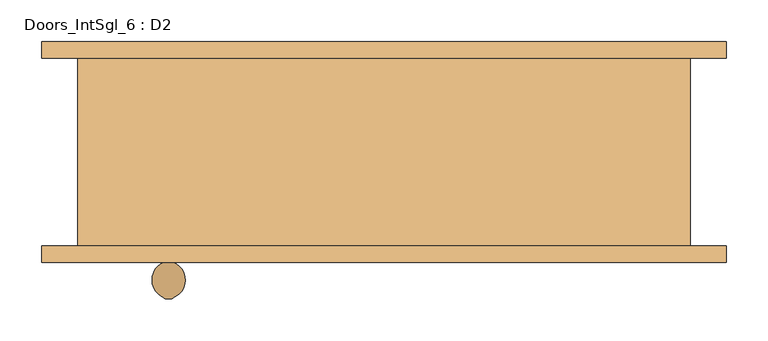
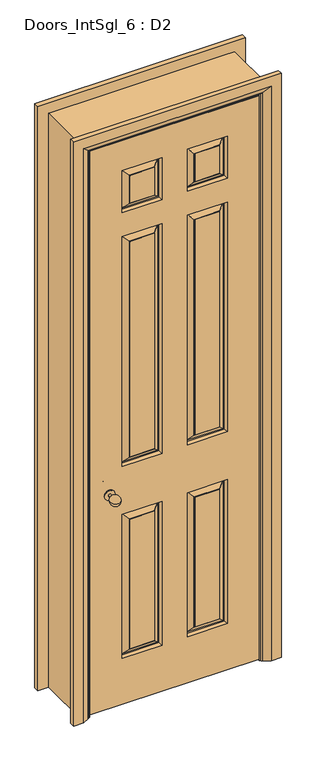
"""IFC4 building model written with IfcOpenShell, lengths in millimetres: door geometry, Doors_IntSgl_6 : D2."""

from ifc_helpers import new_model, si_unit, point, frame, origin, place, context, project, spatial, polyline, circle_curve, ellipse_curve, trimmed, outline, extrude, faceted_brep, source, transform, mapped, element, save
from ifc_brep_helpers import plane_surface, cylinder_surface, revolved_surface, advanced_brep


def doors_intsgl_6_d2_0bf64c77(model_context):
    return source(origin(), model_context, "Body", "SolidModel", [
        advanced_brep(
        [(-253.0, -55.5, 900.0), (-263.0, -55.5, 900.0), (-258.0, -11.062589, 900.0), (-253.0, -70.5, 900.0), (-263.0, -70.5, 900.0), (-278.0, -74.5, 900.0), (-238.0, -74.5, 900.0), (-278.0, -70.5, 900.0), (-238.0, -70.5, 900.0)],
        [
            (0, 1, circle_curve(frame((-258.0, -55.5, 900.0), z_axis=(0.0, 1.0, 0.0), x_axis=(-1.0, 0.0, 0.0)), 5.0)),
            (1, 2, circle_curve(frame((-254.8115138, -33.9213505, 900.0), z_axis=(0.0, 0.0, -1.0), x_axis=(0.0, -1.0, 0.0)), 23.0800654)),
            (2, 0, circle_curve(frame((-261.1884862, -33.9213505, 900.0), z_axis=(0.0, 0.0, -1.0), x_axis=(0.0, -1.0, 0.0)), 23.0800654)),
            (1, 0, circle_curve(frame((-258.0, -55.5, 900.0), z_axis=(0.0, 1.0, 0.0), x_axis=(-1.0, 0.0, 0.0)), 5.0)),
            (0, 3),
            (3, 4, circle_curve(frame((-258.0, -70.5, 900.0), z_axis=(0.0, 1.0, 0.0), x_axis=(-1.0, 0.0, 0.0)), 5.0)),
            (4, 1),
            (4, 3, circle_curve(frame((-258.0, -70.5, 900.0), z_axis=(0.0, 1.0, 0.0), x_axis=(-1.0, 0.0, 0.0)), 5.0)),
            (5, 6, circle_curve(frame((-258.0, -74.5, 900.0), z_axis=(0.0, -1.0, 0.0), x_axis=(1.0, 0.0, 0.0)), 20.0)),
            (6, 5, circle_curve(frame((-258.0, -74.5, 900.0), z_axis=(0.0, -1.0, 0.0), x_axis=(1.0, 0.0, 0.0)), 20.0)),
            (7, 8, circle_curve(frame((-258.0, -70.5, 900.0), z_axis=(0.0, 1.0, 0.0), x_axis=(1.0, 0.0, 0.0)), 20.0)),
            (8, 7, circle_curve(frame((-258.0, -70.5, 900.0), z_axis=(0.0, 1.0, 0.0), x_axis=(1.0, 0.0, 0.0)), 20.0)),
            (5, 7),
            (8, 6),
        ],
        [
            revolved_surface(trimmed(ellipse_curve(frame((-254.8115138, -33.9213505, 900.0), z_axis=(0.0, 0.0, 1.0), x_axis=(0.0, -1.0, 0.0)), 23.0800654, 23.0800654), [point((-258.0, -11.062589, 900.0))], [point((-263.0, -55.5, 900.0))], True, "CARTESIAN"), (-258.0, -70.5, 900.0), (0.0, -1.0, 0.0)),
            cylinder_surface(frame((-258.0, -70.5, 900.0), z_axis=(0.0, -1.0, 0.0), x_axis=(-1.0, 0.0, 0.0)), 5.0),
            plane_surface(frame((-238.0, -74.5, 900.0), z_axis=(0.0, -1.0, 0.0), x_axis=(0.0, 0.0, 1.0))),
            plane_surface(frame((-238.0, -70.5, 900.0), z_axis=(0.0, 1.0, 0.0), x_axis=(0.0, 0.0, -1.0))),
            cylinder_surface(frame((-258.0, -70.5, 900.0), z_axis=(0.0, -1.0, 0.0), x_axis=(1.0, 0.0, 0.0)), 20.0),
        ],
        [
            (0, [[1, 2, 3]]),
            (0, [[-2, 4, -3]]),
            (1, [[-1, 5, 6, 7]]),
            (1, [[-4, -7, 8, -5]]),
            (2, [[9, 10]]),
            (3, [[11, 12], [-6, -8]]),
            (4, [[-9, 13, -12, 14]]),
            (4, [[-10, -14, -11, -13]]),
        ],
    ),
        advanced_brep(
        [(-253.0, -131.5, 900.0), (-258.0, -175.937411, 900.0), (-263.0, -131.5, 900.0), (-263.0, -116.5, 900.0), (-253.0, -116.5, 900.0), (-278.0, -112.5, 900.0), (-238.0, -112.5, 900.0), (-278.0, -116.5, 900.0), (-238.0, -116.5, 900.0)],
        [
            (0, 1, circle_curve(frame((-261.1884862, -153.0786495, 900.0), z_axis=(0.0, 0.0, -1.0), x_axis=(0.0, 1.0, 0.0)), 23.0800654)),
            (1, 2, circle_curve(frame((-254.8115138, -153.0786495, 900.0), z_axis=(0.0, 0.0, -1.0), x_axis=(0.0, 1.0, 0.0)), 23.0800654)),
            (2, 0, circle_curve(frame((-258.0, -131.5, 900.0), z_axis=(0.0, -1.0, 0.0), x_axis=(-1.0, 0.0, 0.0)), 5.0)),
            (0, 2, circle_curve(frame((-258.0, -131.5, 900.0), z_axis=(0.0, -1.0, 0.0), x_axis=(-1.0, 0.0, 0.0)), 5.0)),
            (2, 3),
            (3, 4, circle_curve(frame((-258.0, -116.5, 900.0), z_axis=(0.0, -1.0, 0.0), x_axis=(-1.0, 0.0, 0.0)), 5.0)),
            (4, 0),
            (4, 3, circle_curve(frame((-258.0, -116.5, 900.0), z_axis=(0.0, -1.0, 0.0), x_axis=(-1.0, 0.0, 0.0)), 5.0)),
            (5, 6, circle_curve(frame((-258.0, -112.5, 900.0), z_axis=(0.0, 1.0, 0.0), x_axis=(1.0, 0.0, 0.0)), 20.0)),
            (6, 5, circle_curve(frame((-258.0, -112.5, 900.0), z_axis=(0.0, 1.0, 0.0), x_axis=(1.0, 0.0, 0.0)), 20.0)),
            (7, 8, circle_curve(frame((-258.0, -116.5, 900.0), z_axis=(0.0, -1.0, 0.0), x_axis=(1.0, 0.0, 0.0)), 20.0)),
            (8, 7, circle_curve(frame((-258.0, -116.5, 900.0), z_axis=(0.0, -1.0, 0.0), x_axis=(1.0, 0.0, 0.0)), 20.0)),
            (6, 8),
            (7, 5),
        ],
        [
            revolved_surface(trimmed(ellipse_curve(frame((-254.8115138, -153.0786495, 900.0), z_axis=(0.0, 0.0, -1.0), x_axis=(0.0, 1.0, 0.0)), 23.0800654, 23.0800654), [point((-258.0, -175.937411, 900.0))], [point((-263.0, -131.5, 900.0))], True, "CARTESIAN"), (-258.0, -116.5, 900.0), (0.0, 1.0, 0.0)),
            cylinder_surface(frame((-258.0, -116.5, 900.0), z_axis=(0.0, 1.0, 0.0), x_axis=(-1.0, 0.0, 0.0)), 5.0),
            plane_surface(frame((-238.0, -112.5, 900.0), z_axis=(0.0, 1.0, 0.0), x_axis=(0.0, 0.0, 1.0))),
            plane_surface(frame((-238.0, -116.5, 900.0), z_axis=(0.0, -1.0, 0.0), x_axis=(0.0, 0.0, -1.0))),
            cylinder_surface(frame((-258.0, -116.5, 900.0), z_axis=(0.0, 1.0, 0.0), x_axis=(1.0, 0.0, 0.0)), 20.0),
        ],
        [
            (0, [[1, 2, 3]]),
            (0, [[-1, 4, -2]]),
            (1, [[5, 6, 7, -3]]),
            (1, [[-7, 8, -5, -4]]),
            (2, [[9, 10]]),
            (3, [[11, 12], [-8, -6]]),
            (4, [[13, -11, 14, -10]]),
            (4, [[-14, -12, -13, -9]]),
        ],
    ),
        faceted_brep([(-333.0, -74.5, 2358.0), (333.0, -74.5, 2358.0), (333.0, -74.5, 8.0), (-333.0, -74.5, 8.0), (-50.0, -74.5, 800.0), (-208.0, -74.5, 800.0), (-208.0, -74.5, 200.0), (-50.0, -74.5, 200.0), (208.0, -74.5, 800.0), (50.0, -74.5, 800.0), (50.0, -74.5, 200.0), (208.0, -74.5, 200.0), (-50.0, -74.5, 1958.0), (-208.0, -74.5, 1958.0), (-208.0, -74.5, 1000.0), (-50.0, -74.5, 1000.0), (208.0, -74.5, 1958.0), (50.0, -74.5, 1958.0), (50.0, -74.5, 1000.0), (208.0, -74.5, 1000.0), (-50.0, -74.5, 2233.0), (-208.0, -74.5, 2233.0), (-208.0, -74.5, 2058.0), (-50.0, -74.5, 2058.0), (208.0, -74.5, 2233.0), (50.0, -74.5, 2233.0), (50.0, -74.5, 2058.0), (208.0, -74.5, 2058.0), (-80.0, -74.5, 230.0), (-178.0, -74.5, 230.0), (-178.0, -74.5, 770.0), (-80.0, -74.5, 770.0), (178.0, -74.5, 230.0), (80.0, -74.5, 230.0), (80.0, -74.5, 770.0), (178.0, -74.5, 770.0), (-80.0, -74.5, 1030.0), (-178.0, -74.5, 1030.0), (-178.0, -74.5, 1928.0), (-80.0, -74.5, 1928.0), (178.0, -74.5, 1030.0), (80.0, -74.5, 1030.0), (80.0, -74.5, 1928.0), (178.0, -74.5, 1928.0), (-80.0, -74.5, 2088.0), (-178.0, -74.5, 2088.0), (-178.0, -74.5, 2203.0), (-80.0, -74.5, 2203.0), (178.0, -74.5, 2088.0), (80.0, -74.5, 2088.0), (80.0, -74.5, 2203.0), (178.0, -74.5, 2203.0), (-333.0, -112.5, 2358.0), (-333.0, -112.5, 8.0), (333.0, -112.5, 8.0), (333.0, -112.5, 2358.0), (50.0, -112.5, 800.0), (208.0, -112.5, 800.0), (208.0, -112.5, 200.0), (50.0, -112.5, 200.0), (-208.0, -112.5, 800.0), (-50.0, -112.5, 800.0), (-50.0, -112.5, 200.0), (-208.0, -112.5, 200.0), (50.0, -112.5, 1958.0), (208.0, -112.5, 1958.0), (208.0, -112.5, 1000.0), (50.0, -112.5, 1000.0), (-208.0, -112.5, 1958.0), (-50.0, -112.5, 1958.0), (-50.0, -112.5, 1000.0), (-208.0, -112.5, 1000.0), (50.0, -112.5, 2233.0), (208.0, -112.5, 2233.0), (208.0, -112.5, 2058.0), (50.0, -112.5, 2058.0), (-208.0, -112.5, 2233.0), (-50.0, -112.5, 2233.0), (-50.0, -112.5, 2058.0), (-208.0, -112.5, 2058.0), (80.0, -112.5, 230.0), (178.0, -112.5, 230.0), (178.0, -112.5, 770.0), (80.0, -112.5, 770.0), (-178.0, -112.5, 230.0), (-80.0, -112.5, 230.0), (-80.0, -112.5, 770.0), (-178.0, -112.5, 770.0), (80.0, -112.5, 1030.0), (178.0, -112.5, 1030.0), (178.0, -112.5, 1928.0), (80.0, -112.5, 1928.0), (-178.0, -112.5, 1030.0), (-80.0, -112.5, 1030.0), (-80.0, -112.5, 1928.0), (-178.0, -112.5, 1928.0), (80.0, -112.5, 2088.0), (178.0, -112.5, 2088.0), (178.0, -112.5, 2203.0), (80.0, -112.5, 2203.0), (-178.0, -112.5, 2088.0), (-80.0, -112.5, 2088.0), (-80.0, -112.5, 2203.0), (-178.0, -112.5, 2203.0), (80.0, -111.5, 230.0), (80.0, -111.5, 770.0), (58.0, -97.5, 208.0), (78.0, -111.5, 228.0), (78.0, -111.5, 772.0), (58.0, -97.5, 792.0), (53.0, -97.5, 203.0), (53.0, -97.5, 797.0), (178.0, -111.5, 770.0), (180.0, -111.5, 772.0), (200.0, -97.5, 792.0), (205.0, -97.5, 797.0), (178.0, -111.5, 230.0), (180.0, -111.5, 228.0), (200.0, -97.5, 208.0), (205.0, -97.5, 203.0), (-178.0, -111.5, 230.0), (-178.0, -111.5, 770.0), (-200.0, -97.5, 208.0), (-180.0, -111.5, 228.0), (-180.0, -111.5, 772.0), (-200.0, -97.5, 792.0), (-205.0, -97.5, 203.0), (-205.0, -97.5, 797.0), (-80.0, -111.5, 770.0), (-78.0, -111.5, 772.0), (-58.0, -97.5, 792.0), (-53.0, -97.5, 797.0), (-80.0, -111.5, 230.0), (-78.0, -111.5, 228.0), (-58.0, -97.5, 208.0), (-53.0, -97.5, 203.0), (80.0, -111.5, 1030.0), (80.0, -111.5, 1928.0), (58.0, -97.5, 1008.0), (78.0, -111.5, 1028.0), (78.0, -111.5, 1930.0), (58.0, -97.5, 1950.0), (53.0, -97.5, 1003.0), (53.0, -97.5, 1955.0), (178.0, -111.5, 1928.0), (180.0, -111.5, 1930.0), (200.0, -97.5, 1950.0), (205.0, -97.5, 1955.0), (178.0, -111.5, 1030.0), (180.0, -111.5, 1028.0), (200.0, -97.5, 1008.0), (205.0, -97.5, 1003.0), (-178.0, -111.5, 1030.0), (-178.0, -111.5, 1928.0), (-200.0, -97.5, 1008.0), (-180.0, -111.5, 1028.0), (-180.0, -111.5, 1930.0), (-200.0, -97.5, 1950.0), (-205.0, -97.5, 1003.0), (-205.0, -97.5, 1955.0), (-80.0, -111.5, 1928.0), (-78.0, -111.5, 1930.0), (-58.0, -97.5, 1950.0), (-53.0, -97.5, 1955.0), (-80.0, -111.5, 1030.0), (-78.0, -111.5, 1028.0), (-58.0, -97.5, 1008.0), (-53.0, -97.5, 1003.0), (80.0, -111.5, 2088.0), (80.0, -111.5, 2203.0), (58.0, -97.5, 2066.0), (78.0, -111.5, 2086.0), (78.0, -111.5, 2205.0), (58.0, -97.5, 2225.0), (53.0, -97.5, 2061.0), (53.0, -97.5, 2230.0), (178.0, -111.5, 2203.0), (180.0, -111.5, 2205.0), (200.0, -97.5, 2225.0), (205.0, -97.5, 2230.0), (178.0, -111.5, 2088.0), (180.0, -111.5, 2086.0), (200.0, -97.5, 2066.0), (205.0, -97.5, 2061.0), (-178.0, -111.5, 2088.0), (-178.0, -111.5, 2203.0), (-200.0, -97.5, 2066.0), (-180.0, -111.5, 2086.0), (-180.0, -111.5, 2205.0), (-200.0, -97.5, 2225.0), (-205.0, -97.5, 2061.0), (-205.0, -97.5, 2230.0), (-80.0, -111.5, 2203.0), (-78.0, -111.5, 2205.0), (-58.0, -97.5, 2225.0), (-53.0, -97.5, 2230.0), (-80.0, -111.5, 2088.0), (-78.0, -111.5, 2086.0), (-58.0, -97.5, 2066.0), (-53.0, -97.5, 2061.0), (-80.0, -75.5, 230.0), (-80.0, -75.5, 770.0), (-58.0, -89.5, 208.0), (-78.0, -75.5, 228.0), (-78.0, -75.5, 772.0), (-58.0, -89.5, 792.0), (-53.0, -89.5, 203.0), (-53.0, -89.5, 797.0), (-178.0, -75.5, 770.0), (-180.0, -75.5, 772.0), (-200.0, -89.5, 792.0), (-205.0, -89.5, 797.0), (-178.0, -75.5, 230.0), (-180.0, -75.5, 228.0), (-200.0, -89.5, 208.0), (-205.0, -89.5, 203.0), (178.0, -75.5, 230.0), (178.0, -75.5, 770.0), (200.0, -89.5, 208.0), (180.0, -75.5, 228.0), (180.0, -75.5, 772.0), (200.0, -89.5, 792.0), (205.0, -89.5, 203.0), (205.0, -89.5, 797.0), (80.0, -75.5, 770.0), (78.0, -75.5, 772.0), (58.0, -89.5, 792.0), (53.0, -89.5, 797.0), (80.0, -75.5, 230.0), (78.0, -75.5, 228.0), (58.0, -89.5, 208.0), (53.0, -89.5, 203.0), (-80.0, -75.5, 1030.0), (-80.0, -75.5, 1928.0), (-58.0, -89.5, 1008.0), (-78.0, -75.5, 1028.0), (-78.0, -75.5, 1930.0), (-58.0, -89.5, 1950.0), (-53.0, -89.5, 1003.0), (-53.0, -89.5, 1955.0), (-178.0, -75.5, 1928.0), (-180.0, -75.5, 1930.0), (-200.0, -89.5, 1950.0), (-205.0, -89.5, 1955.0), (-178.0, -75.5, 1030.0), (-180.0, -75.5, 1028.0), (-200.0, -89.5, 1008.0), (-205.0, -89.5, 1003.0), (178.0, -75.5, 1030.0), (178.0, -75.5, 1928.0), (200.0, -89.5, 1008.0), (180.0, -75.5, 1028.0), (180.0, -75.5, 1930.0), (200.0, -89.5, 1950.0), (205.0, -89.5, 1003.0), (205.0, -89.5, 1955.0), (80.0, -75.5, 1928.0), (78.0, -75.5, 1930.0), (58.0, -89.5, 1950.0), (53.0, -89.5, 1955.0), (80.0, -75.5, 1030.0), (78.0, -75.5, 1028.0), (58.0, -89.5, 1008.0), (53.0, -89.5, 1003.0), (-80.0, -75.5, 2088.0), (-80.0, -75.5, 2203.0), (-58.0, -89.5, 2066.0), (-78.0, -75.5, 2086.0), (-78.0, -75.5, 2205.0), (-58.0, -89.5, 2225.0), (-53.0, -89.5, 2061.0), (-53.0, -89.5, 2230.0), (-178.0, -75.5, 2203.0), (-180.0, -75.5, 2205.0), (-200.0, -89.5, 2225.0), (-205.0, -89.5, 2230.0), (-178.0, -75.5, 2088.0), (-180.0, -75.5, 2086.0), (-200.0, -89.5, 2066.0), (-205.0, -89.5, 2061.0), (178.0, -75.5, 2088.0), (178.0, -75.5, 2203.0), (200.0, -89.5, 2066.0), (180.0, -75.5, 2086.0), (180.0, -75.5, 2205.0), (200.0, -89.5, 2225.0), (205.0, -89.5, 2061.0), (205.0, -89.5, 2230.0), (80.0, -75.5, 2203.0), (78.0, -75.5, 2205.0), (58.0, -89.5, 2225.0), (53.0, -89.5, 2230.0), (80.0, -75.5, 2088.0), (78.0, -75.5, 2086.0), (58.0, -89.5, 2066.0), (53.0, -89.5, 2061.0)], [[[0, 1, 2, 3], [4, 5, 6, 7], [8, 9, 10, 11], [12, 13, 14, 15], [16, 17, 18, 19], [20, 21, 22, 23], [24, 25, 26, 27]], [[28, 29, 30, 31]], [[32, 33, 34, 35]], [[36, 37, 38, 39]], [[40, 41, 42, 43]], [[44, 45, 46, 47]], [[48, 49, 50, 51]], [[52, 53, 54, 55], [56, 57, 58, 59], [60, 61, 62, 63], [64, 65, 66, 67], [68, 69, 70, 71], [72, 73, 74, 75], [76, 77, 78, 79]], [[80, 81, 82, 83]], [[84, 85, 86, 87]], [[88, 89, 90, 91]], [[92, 93, 94, 95]], [[96, 97, 98, 99]], [[100, 101, 102, 103]], [[3, 53, 52, 0]], [[2, 54, 53, 3]], [[1, 55, 54, 2]], [[0, 52, 55, 1]], [[104, 80, 83, 105]], [[106, 107, 108, 109]], [[56, 59, 110, 111]], [[83, 82, 112, 105]], [[108, 113, 114, 109]], [[111, 115, 57, 56]], [[82, 81, 116, 112]], [[113, 117, 118, 114]], [[115, 119, 58, 57]], [[104, 116, 81, 80]], [[107, 117, 113, 108], [105, 112, 116, 104]], [[106, 118, 117, 107]], [[110, 119, 115, 111], [109, 114, 118, 106]], [[59, 58, 119, 110]], [[120, 84, 87, 121]], [[122, 123, 124, 125]], [[60, 63, 126, 127]], [[87, 86, 128, 121]], [[124, 129, 130, 125]], [[127, 131, 61, 60]], [[86, 85, 132, 128]], [[129, 133, 134, 130]], [[131, 135, 62, 61]], [[120, 132, 85, 84]], [[123, 133, 129, 124], [121, 128, 132, 120]], [[122, 134, 133, 123]], [[126, 135, 131, 127], [125, 130, 134, 122]], [[63, 62, 135, 126]], [[136, 88, 91, 137]], [[138, 139, 140, 141]], [[64, 67, 142, 143]], [[91, 90, 144, 137]], [[140, 145, 146, 141]], [[143, 147, 65, 64]], [[90, 89, 148, 144]], [[145, 149, 150, 146]], [[147, 151, 66, 65]], [[136, 148, 89, 88]], [[139, 149, 145, 140], [137, 144, 148, 136]], [[138, 150, 149, 139]], [[142, 151, 147, 143], [141, 146, 150, 138]], [[67, 66, 151, 142]], [[152, 92, 95, 153]], [[154, 155, 156, 157]], [[68, 71, 158, 159]], [[95, 94, 160, 153]], [[156, 161, 162, 157]], [[159, 163, 69, 68]], [[94, 93, 164, 160]], [[161, 165, 166, 162]], [[163, 167, 70, 69]], [[152, 164, 93, 92]], [[155, 165, 161, 156], [153, 160, 164, 152]], [[154, 166, 165, 155]], [[158, 167, 163, 159], [157, 162, 166, 154]], [[71, 70, 167, 158]], [[168, 96, 99, 169]], [[170, 171, 172, 173]], [[72, 75, 174, 175]], [[99, 98, 176, 169]], [[172, 177, 178, 173]], [[175, 179, 73, 72]], [[98, 97, 180, 176]], [[177, 181, 182, 178]], [[179, 183, 74, 73]], [[168, 180, 97, 96]], [[171, 181, 177, 172], [169, 176, 180, 168]], [[170, 182, 181, 171]], [[174, 183, 179, 175], [173, 178, 182, 170]], [[75, 74, 183, 174]], [[184, 100, 103, 185]], [[186, 187, 188, 189]], [[76, 79, 190, 191]], [[103, 102, 192, 185]], [[188, 193, 194, 189]], [[191, 195, 77, 76]], [[102, 101, 196, 192]], [[193, 197, 198, 194]], [[195, 199, 78, 77]], [[184, 196, 101, 100]], [[187, 197, 193, 188], [185, 192, 196, 184]], [[186, 198, 197, 187]], [[190, 199, 195, 191], [189, 194, 198, 186]], [[79, 78, 199, 190]], [[200, 28, 31, 201]], [[202, 203, 204, 205]], [[4, 7, 206, 207]], [[31, 30, 208, 201]], [[204, 209, 210, 205]], [[207, 211, 5, 4]], [[30, 29, 212, 208]], [[209, 213, 214, 210]], [[211, 215, 6, 5]], [[200, 212, 29, 28]], [[203, 213, 209, 204], [201, 208, 212, 200]], [[202, 214, 213, 203]], [[206, 215, 211, 207], [205, 210, 214, 202]], [[7, 6, 215, 206]], [[216, 32, 35, 217]], [[218, 219, 220, 221]], [[8, 11, 222, 223]], [[35, 34, 224, 217]], [[220, 225, 226, 221]], [[223, 227, 9, 8]], [[34, 33, 228, 224]], [[225, 229, 230, 226]], [[227, 231, 10, 9]], [[216, 228, 33, 32]], [[219, 229, 225, 220], [217, 224, 228, 216]], [[218, 230, 229, 219]], [[222, 231, 227, 223], [221, 226, 230, 218]], [[11, 10, 231, 222]], [[232, 36, 39, 233]], [[234, 235, 236, 237]], [[12, 15, 238, 239]], [[39, 38, 240, 233]], [[236, 241, 242, 237]], [[239, 243, 13, 12]], [[38, 37, 244, 240]], [[241, 245, 246, 242]], [[243, 247, 14, 13]], [[232, 244, 37, 36]], [[235, 245, 241, 236], [233, 240, 244, 232]], [[234, 246, 245, 235]], [[238, 247, 243, 239], [237, 242, 246, 234]], [[15, 14, 247, 238]], [[248, 40, 43, 249]], [[250, 251, 252, 253]], [[16, 19, 254, 255]], [[43, 42, 256, 249]], [[252, 257, 258, 253]], [[255, 259, 17, 16]], [[42, 41, 260, 256]], [[257, 261, 262, 258]], [[259, 263, 18, 17]], [[248, 260, 41, 40]], [[251, 261, 257, 252], [249, 256, 260, 248]], [[250, 262, 261, 251]], [[254, 263, 259, 255], [253, 258, 262, 250]], [[19, 18, 263, 254]], [[264, 44, 47, 265]], [[266, 267, 268, 269]], [[20, 23, 270, 271]], [[47, 46, 272, 265]], [[268, 273, 274, 269]], [[271, 275, 21, 20]], [[46, 45, 276, 272]], [[273, 277, 278, 274]], [[275, 279, 22, 21]], [[264, 276, 45, 44]], [[267, 277, 273, 268], [265, 272, 276, 264]], [[266, 278, 277, 267]], [[270, 279, 275, 271], [269, 274, 278, 266]], [[23, 22, 279, 270]], [[280, 48, 51, 281]], [[282, 283, 284, 285]], [[24, 27, 286, 287]], [[51, 50, 288, 281]], [[284, 289, 290, 285]], [[287, 291, 25, 24]], [[50, 49, 292, 288]], [[289, 293, 294, 290]], [[291, 295, 26, 25]], [[280, 292, 49, 48]], [[283, 293, 289, 284], [281, 288, 292, 280]], [[282, 294, 293, 283]], [[286, 295, 291, 287], [285, 290, 294, 282]], [[27, 26, 295, 286]]]),
        faceted_brep([(-335.0, -112.5, 0.0), (-367.0, -112.5, 0.0), (-367.0, 112.5, 0.0), (-335.0, 112.5, 0.0), (-335.0, 112.5, 2360.0), (-335.0, -112.5, 2360.0), (-367.0, 112.5, 2392.0), (-367.0, -112.5, 2392.0), (335.0, -112.5, 0.0), (335.0, 112.5, 0.0), (367.0, 112.5, 0.0), (367.0, -112.5, 0.0), (335.0, -112.5, 2360.0), (367.0, -112.5, 2392.0), (367.0, 112.5, 2392.0), (335.0, 112.5, 2360.0)], [[[0, 1, 2, 3]], [[3, 4, 5, 0]], [[2, 6, 4, 3]], [[1, 7, 6, 2]], [[0, 5, 7, 1]], [[8, 9, 10, 11]], [[12, 8, 11, 13]], [[13, 11, 10, 14]], [[14, 10, 9, 15]], [[15, 9, 8, 12]], [[4, 15, 12, 5]], [[6, 14, 15, 4]], [[7, 13, 14, 6]], [[5, 12, 13, 7]]]),
        extrude(outline(polyline([(0.0, -316.0), (2341.0, -316.0), (2341.0, 316.0), (0.0, 316.0), (0.0, 335.0), (2360.0, 335.0), (2360.0, -335.0), (0.0, -335.0), (0.0, -316.0)])), frame((0.0, -72.5, 0.0), z_axis=(0.0, 1.0, 0.0), x_axis=(0.0, 0.0, 1.0)), (0.0, 0.0, 1.0), 32.0),
        advanced_brep(
        [(-410.0, 132.5, 0.0), (-370.0, 132.5, 0.0), (-344.0, 118.5, 0.0), (-340.0, 112.5, 0.0), (-410.0, 112.5, 0.0), (-410.0, 112.5, 2435.0), (-410.0, 132.5, 2435.0), (-340.0, 112.5, 2365.0), (340.0, 112.5, 2365.0), (340.0, 112.5, 0.0), (410.0, 112.5, 0.0), (410.0, 112.5, 2435.0), (-344.0, 118.5, 2369.0), (-370.0, 132.5, 2395.0), (410.0, 132.5, 2435.0), (410.0, 132.5, 0.0), (370.0, 132.5, 0.0), (370.0, 132.5, 2395.0), (344.0, 118.5, 0.0), (344.0, 118.5, 2369.0)],
        [
            (0, 1),
            (1, 2),
            (2, 3, circle_curve(frame((-348.0, 111.5, 0.0), z_axis=(0.0, 0.0, -1.0), x_axis=(-1.0, 0.0, 0.0)), 8.0622577)),
            (3, 4),
            (4, 0),
            (4, 5),
            (5, 6),
            (6, 0),
            (3, 7),
            (7, 8),
            (8, 9),
            (9, 10),
            (10, 11),
            (11, 5),
            (2, 12),
            (12, 7, ellipse_curve(frame((-348.0, 111.5, 2373.0), z_axis=(-0.7071067811865475, 0.0, -0.7071067811865475), x_axis=(0.7071067811865474, 0.0, -0.7071067811865476)), 11.4017543, 8.0622577)),
            (1, 13),
            (13, 12),
            (6, 14),
            (14, 15),
            (15, 16),
            (16, 17),
            (17, 13),
            (10, 15),
            (14, 11),
            (9, 18, circle_curve(frame((348.0, 111.5, 0.0), z_axis=(0.0, 0.0, -1.0), x_axis=(1.0, 0.0, 0.0)), 8.0622577)),
            (18, 16),
            (19, 18),
            (8, 19, ellipse_curve(frame((348.0, 111.5, 2373.0), z_axis=(0.7071067811865475, 0.0, -0.7071067811865475), x_axis=(0.7071067811865474, 0.0, 0.7071067811865476)), 11.4017543, 8.0622577)),
            (19, 17),
            (12, 19),
        ],
        [
            plane_surface(frame((-340.0, 112.5, 0.0), z_axis=(0.0, 0.0, -1.0), x_axis=(0.0, 1.0, 0.0))),
            plane_surface(frame((-410.0, 132.5, 0.0), z_axis=(-1.0, 0.0, 0.0), x_axis=(0.0, 0.0, 1.0))),
            plane_surface(frame((-410.0, 112.5, 0.0), z_axis=(0.0, -1.0, 0.0), x_axis=(0.0, 0.0, 1.0))),
            cylinder_surface(frame((-348.0, 111.5, 0.0), z_axis=(0.0, 0.0, -1.0), x_axis=(-1.0, 0.0, 0.0)), 8.0622577),
            plane_surface(frame((-344.0, 118.5, 0.0), z_axis=(0.4740998230350183, 0.8804710999221749, 0.0), x_axis=(0.0, 0.0, 1.0))),
            plane_surface(frame((-370.0, 132.5, 0.0), z_axis=(0.0, 1.0, 0.0), x_axis=(0.0, 0.0, 1.0))),
            plane_surface(frame((410.0, 132.5, 2435.0), z_axis=(1.0, 0.0, 0.0), x_axis=(0.0, 0.0, -1.0))),
            plane_surface(frame((340.0, 112.5, 0.0), z_axis=(0.0, 0.0, -1.0), x_axis=(0.0, 1.0, 0.0))),
            cylinder_surface(frame((348.0, 111.5, 2365.0), z_axis=(0.0, 0.0, 1.0), x_axis=(1.0, 0.0, 0.0)), 8.0622577),
            plane_surface(frame((344.0, 118.5, 2369.0), z_axis=(-0.4740998230350183, 0.8804710999221749, 0.0), x_axis=(0.0, 0.0, -1.0))),
            plane_surface(frame((-410.0, 132.5, 2435.0), z_axis=(0.0, 0.0, 1.0), x_axis=(1.0, 0.0, 0.0))),
            cylinder_surface(frame((-340.0, 111.5, 2373.0), z_axis=(-1.0, 0.0, 0.0), x_axis=(0.0, 0.0, 1.0)), 8.0622577),
            plane_surface(frame((-344.0, 118.5, 2369.0), z_axis=(0.0, 0.8804710999221749, -0.4740998230350183), x_axis=(1.0, 0.0, 0.0))),
        ],
        [
            (0, [[1, 2, 3, 4, 5]]),
            (1, [[6, 7, 8, -5]]),
            (2, [[9, 10, 11, 12, 13, 14, -6, -4]]),
            (3, [[15, 16, -9, -3]]),
            (4, [[17, 18, -15, -2]]),
            (5, [[-8, 19, 20, 21, 22, 23, -17, -1]]),
            (6, [[-13, 24, -20, 25]]),
            (7, [[-24, -12, 26, 27, -21]]),
            (8, [[28, -26, -11, 29]]),
            (9, [[-22, -27, -28, 30]]),
            (10, [[-14, -25, -19, -7]]),
            (11, [[31, -29, -10, -16]]),
            (12, [[-23, -30, -31, -18]]),
        ],
    ),
        advanced_brep(
        [(410.0, -132.5, 0.0), (370.0, -132.5, 0.0), (344.0, -118.5, 0.0), (340.0, -112.5, 0.0), (410.0, -112.5, 0.0), (410.0, -112.5, 2435.0), (410.0, -132.5, 2435.0), (340.0, -112.5, 2365.0), (-340.0, -112.5, 2365.0), (-340.0, -112.5, 0.0), (-410.0, -112.5, 0.0), (-410.0, -112.5, 2435.0), (344.0, -118.5, 2369.0), (370.0, -132.5, 2395.0), (-410.0, -132.5, 2435.0), (-410.0, -132.5, 0.0), (-370.0, -132.5, 0.0), (-370.0, -132.5, 2395.0), (-344.0, -118.5, 0.0), (-344.0, -118.5, 2369.0)],
        [
            (0, 1),
            (1, 2),
            (2, 3, circle_curve(frame((348.0, -111.5, 0.0), z_axis=(0.0, 0.0, -1.0), x_axis=(1.0, 0.0, 0.0)), 8.0622577)),
            (3, 4),
            (4, 0),
            (4, 5),
            (5, 6),
            (6, 0),
            (3, 7),
            (7, 8),
            (8, 9),
            (9, 10),
            (10, 11),
            (11, 5),
            (2, 12),
            (12, 7, ellipse_curve(frame((348.0, -111.5, 2373.0), z_axis=(0.7071067811865475, 0.0, -0.7071067811865475), x_axis=(-0.7071067811865474, 0.0, -0.7071067811865476)), 11.4017543, 8.0622577)),
            (1, 13),
            (13, 12),
            (6, 14),
            (14, 15),
            (15, 16),
            (16, 17),
            (17, 13),
            (10, 15),
            (14, 11),
            (9, 18, circle_curve(frame((-348.0, -111.5, 0.0), z_axis=(0.0, 0.0, -1.0), x_axis=(-1.0, 0.0, 0.0)), 8.0622577)),
            (18, 16),
            (19, 18),
            (8, 19, ellipse_curve(frame((-348.0, -111.5, 2373.0), z_axis=(-0.7071067811865475, 0.0, -0.7071067811865475), x_axis=(-0.7071067811865474, 0.0, 0.7071067811865476)), 11.4017543, 8.0622577)),
            (19, 17),
            (12, 19),
        ],
        [
            plane_surface(frame((340.0, -112.5, 0.0), z_axis=(0.0, 0.0, -1.0), x_axis=(0.0, -1.0, 0.0))),
            plane_surface(frame((410.0, -132.5, 0.0), z_axis=(1.0, 0.0, 0.0), x_axis=(0.0, 0.0, 1.0))),
            plane_surface(frame((410.0, -112.5, 0.0), z_axis=(0.0, 1.0, 0.0), x_axis=(0.0, 0.0, 1.0))),
            cylinder_surface(frame((348.0, -111.5, 0.0), z_axis=(0.0, 0.0, -1.0), x_axis=(1.0, 0.0, 0.0)), 8.0622577),
            plane_surface(frame((344.0, -118.5, 0.0), z_axis=(-0.4740998230350183, -0.8804710999221749, 0.0), x_axis=(0.0, 0.0, 1.0))),
            plane_surface(frame((370.0, -132.5, 0.0), z_axis=(0.0, -1.0, 0.0), x_axis=(0.0, 0.0, 1.0))),
            plane_surface(frame((-410.0, -132.5, 2435.0), z_axis=(-1.0, 0.0, 0.0), x_axis=(0.0, 0.0, -1.0))),
            plane_surface(frame((-340.0, -112.5, 0.0), z_axis=(0.0, 0.0, -1.0), x_axis=(0.0, -1.0, 0.0))),
            cylinder_surface(frame((-348.0, -111.5, 2365.0), z_axis=(0.0, 0.0, 1.0), x_axis=(-1.0, 0.0, 0.0)), 8.0622577),
            plane_surface(frame((-344.0, -118.5, 2369.0), z_axis=(0.4740998230350183, -0.8804710999221749, 0.0), x_axis=(0.0, 0.0, -1.0))),
            plane_surface(frame((410.0, -132.5, 2435.0), z_axis=(0.0, 0.0, 1.0), x_axis=(-1.0, 0.0, 0.0))),
            cylinder_surface(frame((340.0, -111.5, 2373.0), z_axis=(1.0, 0.0, 0.0), x_axis=(0.0, 0.0, 1.0)), 8.0622577),
            plane_surface(frame((344.0, -118.5, 2369.0), z_axis=(0.0, -0.8804710999221749, -0.4740998230350183), x_axis=(-1.0, 0.0, 0.0))),
        ],
        [
            (0, [[1, 2, 3, 4, 5]]),
            (1, [[6, 7, 8, -5]]),
            (2, [[9, 10, 11, 12, 13, 14, -6, -4]]),
            (3, [[15, 16, -9, -3]]),
            (4, [[17, 18, -15, -2]]),
            (5, [[-8, 19, 20, 21, 22, 23, -17, -1]]),
            (6, [[-13, 24, -20, 25]]),
            (7, [[-24, -12, 26, 27, -21]]),
            (8, [[28, -26, -11, 29]]),
            (9, [[-22, -27, -28, 30]]),
            (10, [[-14, -25, -19, -7]]),
            (11, [[31, -29, -10, -16]]),
            (12, [[-23, -30, -31, -18]]),
        ],
    ),
    ])


if __name__ == "__main__":
    model = new_model("IFC4")
    model_context = context("Model", 3, world=origin())
    ifc_project = project(units=[si_unit("LENGTHUNIT", "METRE", prefix="MILLI")], contexts=[model_context])
    site = spatial("IfcSite", under=ifc_project)
    building = spatial("IfcBuilding", under=site)
    placement = place(None, origin())
    doors_intsgl_6_d2_shape = doors_intsgl_6_d2_0bf64c77(model_context)
    element("IfcDoor", 1, ObjectType="Doors_IntSgl_6 : D2", at=placement, inside=building, context=model_context, shape_type="MappedRepresentation", body=[
        mapped(doors_intsgl_6_d2_shape, transform((0.0, 0.0, 0.0), x_axis=(1.0, 0.0, 0.0), y_axis=(0.0, 1.0, 0.0), z_axis=(0.0, 0.0, 1.0))),
    ])
    save(model, "model.ifc")

# Revit data of these elements
# Type "Doors_IntSgl_6 : D2"
#   Type Mark = "50"
#   Type Comments = "Internal Single"
#   Operation = "SingleSwingRight"
#   Construction Type Id = "MDOOR"
#   Manufacturer = "Revit"
#   Keynote = "L20"
#   Description = "Internal Single Door"
#   Analytic Construction = "Metal"
#   UnderCut = 8 mm
#   Tolerance = 2 mm
#   Thickness = 38 mm
#   Structural Tolerance = 8 mm
#   StopDepth = 32 mm
#   Stop Thickness = 19 mm
#   Stile Top Rail = 125 mm
#   Stile Shutting = 125 mm
#   Stile Muntin Rail = 100 mm
#   Stile Lock Rail = 200 mm
#   Stile Intermediate/Frieze = 100 mm
#   Stile Hanging = 125 mm
#   Stile Bottom Rail = 200 mm
#   Rough Width = 750 mm
#   Rough Height = 2400 mm
#   Height to Top Lock Rail = 1000 mm
#   Heat Transfer Coefficient (U) = 3.7021 W/(m²·K)
#   Handle Z Distance = 900 mm
#   Handle X Distance = 75 mm
#   Frame Thickness = 32 mm
#   Door Panel Width = 666 mm
#   Height = 2400 mm
#   Width = 750 mm
#   Door Panel Thickness = 38 mm
#   Door Panel Offset = 0 mm
#   Door Panel Height = 2350 mm
#   Architrave Setback = 5 mm
#   Vis - Ironmongery = yes
#   Define Thermal Properties by = 1
#   Material Ironmongery = Door - Handle
#   Material Frame = Door - Frame/Mullion
#   Material Door = Door - Panel
#   Material Architrave = Door - Architrave
#   Visual Light Transmittance = 0
#   Solar Heat Gain Coefficient = 0
#   Function = (empty or 0)
#   Wall Closure = (empty or 0)
# Element 1 (IfcDoor, "Doors_IntSgl_6 : D2")
#   Materials on its faces: "Door - Panel", "Door - Architrave", "Door - Frame/Mullion", "Door - Handle"
# Materials
#   "Door - Handle": colour RGB 247 247 247, transparency 0
#   "Door - Frame/Mullion": class "Wood", colour RGB 212 179 113, transparency 0
#   "Door - Panel": class "Wood", colour RGB 154 90 5, transparency 0
#   "Door - Architrave": class "Wood", colour RGB 154 90 5, transparency 0
